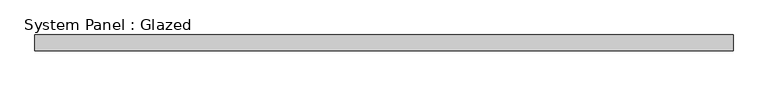
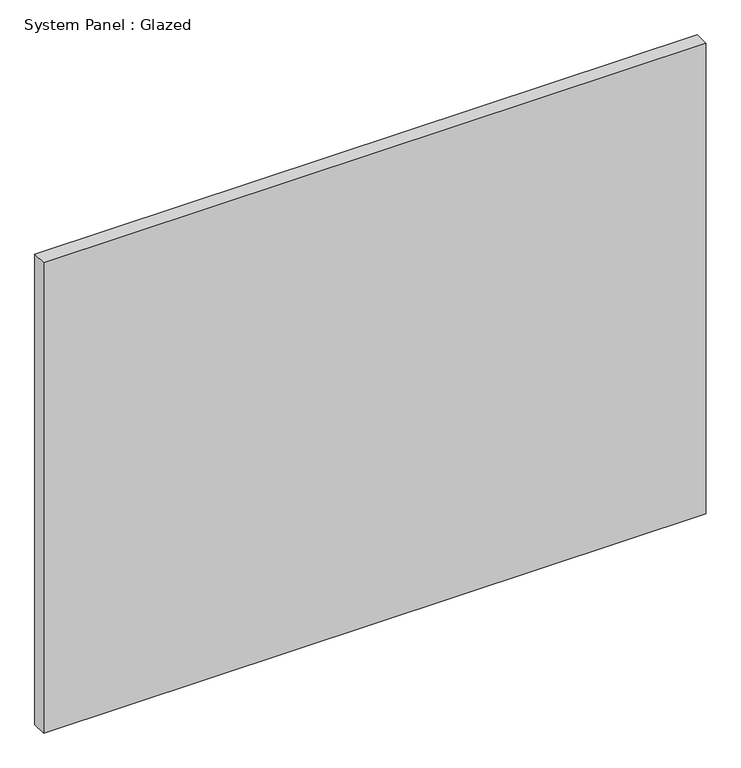
"""IFC4 building model written with IfcOpenShell, lengths in millimetres: plate geometry, System Panel : Glazed."""

from ifc_helpers import new_model, si_unit, origin, origin_with_axes, place, context, project, spatial, polyline, outline, extrude, source, transform, mapped, element, save


def system_panel_glazed_36bafcef(model_context):
    return source(origin(), model_context, "Body", "SweptSolid", [
        extrude(outline(polyline([(565.1500001, 19.05), (-565.1500001, 19.05), (-565.1500001, 44.45), (565.1500001, 44.45), (565.1500001, 19.05)])), origin_with_axes(), (0.0, 0.0, 1.0), 847.5210507),
    ])


if __name__ == "__main__":
    model = new_model("IFC4")
    model_context = context("Model", 3, world=origin())
    ifc_project = project(units=[si_unit("LENGTHUNIT", "METRE", prefix="MILLI")], contexts=[model_context])
    site = spatial("IfcSite", under=ifc_project)
    building = spatial("IfcBuilding", under=site)
    placement = place(None, origin())
    system_panel_glazed_shape = system_panel_glazed_36bafcef(model_context)
    element("IfcPlate", 1, ObjectType="System Panel : Glazed", at=placement, inside=building, context=model_context, shape_type="MappedRepresentation", body=[
        mapped(system_panel_glazed_shape, transform((0.0, 0.0, 0.0), x_axis=(1.0, 0.0, 0.0), y_axis=(0.0, 1.0, 0.0), z_axis=(0.0, 0.0, 1.0))),
    ])
    save(model, "model.ifc")

# Revit data of these elements
# Type "System Panel : Glazed"
#   Construction Type Id = "GSP4R"
#   Analytic Construction = "1/8 in Pilkington single glazing"
#   Visual Light Transmittance = 0.9
#   Solar Heat Gain Coefficient = 0.86
#   Heat Transfer Coefficient (U) = 1.18115 BTU/(h·ft²·°F)
#   Define Thermal Properties by = 1
# Element 1 (IfcPlate, "System Panel : Glazed")
#   Materials on its faces: "Glass"
# Materials
#   "Glass": class "Glass", colour RGB 0 128 192, transparency 0.75, Description = "Soda Lime Glass", Cost = 0
